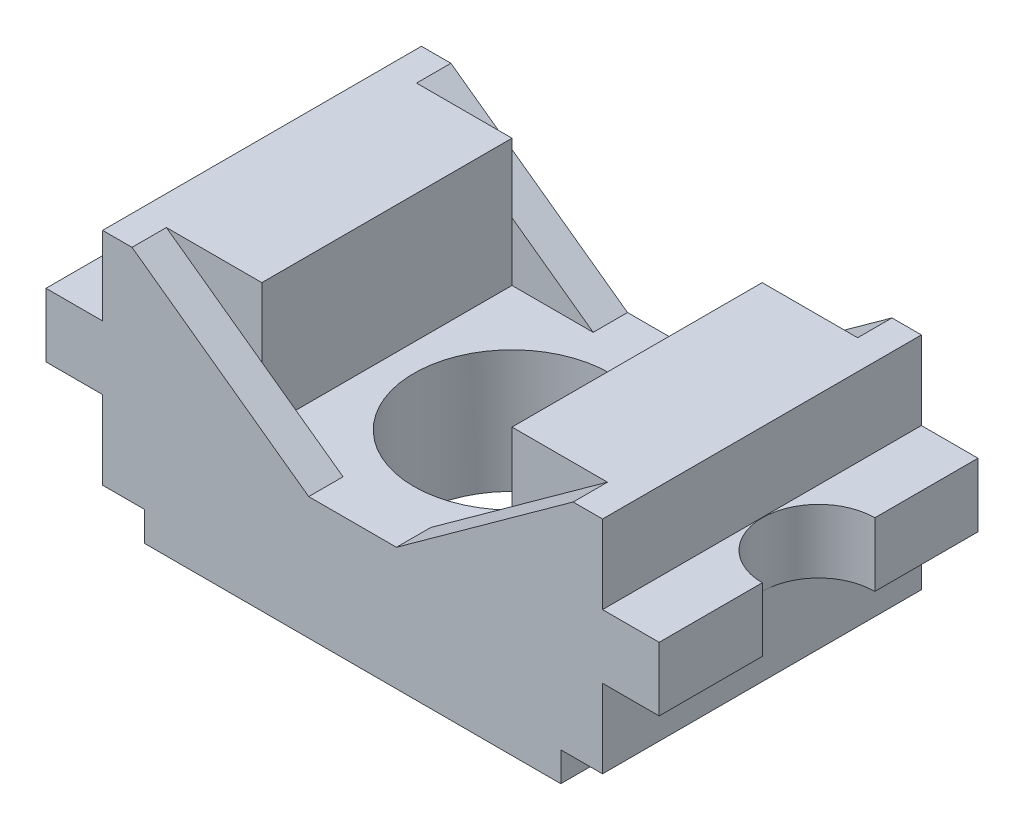
ISO-10303-21;
HEADER;
FILE_DESCRIPTION(('STEP AP214'),'2;1');
FILE_NAME('part.step','',(''),(''),'','','');
FILE_SCHEMA(('AUTOMOTIVE_DESIGN { 1 0 10303 214 1 1 1 1 }'));
ENDSEC;
DATA;
#1=APPLICATION_CONTEXT('core data for automotive mechanical design processes');
#2=APPLICATION_PROTOCOL_DEFINITION('international standard','automotive_design',2000,#1);
#3=PRODUCT_CONTEXT('',#1,'mechanical');
#4=PRODUCT('Part','Part','',(#3));
#5=PRODUCT_RELATED_PRODUCT_CATEGORY('part','',(#4));
#6=PRODUCT_DEFINITION_FORMATION('','',#4);
#7=PRODUCT_DEFINITION_CONTEXT('part definition',#1,'design');
#8=PRODUCT_DEFINITION('design','',#6,#7);
#9=PRODUCT_DEFINITION_SHAPE('','',#8);
#10=(LENGTH_UNIT() NAMED_UNIT(*) SI_UNIT(.MILLI.,.METRE.));
#11=(NAMED_UNIT(*) PLANE_ANGLE_UNIT() SI_UNIT($,.RADIAN.));
#12=(NAMED_UNIT(*) SI_UNIT($,.STERADIAN.) SOLID_ANGLE_UNIT());
#13=UNCERTAINTY_MEASURE_WITH_UNIT(LENGTH_MEASURE(1.E-05),#10,'distance_accuracy_value','');
#14=(GEOMETRIC_REPRESENTATION_CONTEXT(3) GLOBAL_UNCERTAINTY_ASSIGNED_CONTEXT((#13)) GLOBAL_UNIT_ASSIGNED_CONTEXT((#10,
#11,#12)) REPRESENTATION_CONTEXT('',''));
#15=CARTESIAN_POINT('',(0.,0.,0.));
#16=DIRECTION('',(0.,0.,1.));
#17=DIRECTION('',(1.,0.,0.));
#18=AXIS2_PLACEMENT_3D('',#15,#16,#17);
#19=CARTESIAN_POINT('',(62.5,22.,-65.));
#20=DIRECTION('',(1.,0.,0.));
#21=DIRECTION('',(0.,0.,-1.));
#22=AXIS2_PLACEMENT_3D('',#19,#20,#21);
#23=PLANE('',#22);
#24=DIRECTION('',(0.,1.,0.));
#25=VECTOR('',#24,1.);
#26=CARTESIAN_POINT('',(62.5,-6.00000000000003,-43.9726799835102));
#27=LINE('',#26,#25);
#28=CARTESIAN_POINT('',(62.5,22.,-43.9726799835102));
#29=VERTEX_POINT('',#28);
#30=CARTESIAN_POINT('',(62.5,35.,-43.9726799835102));
#31=VERTEX_POINT('',#30);
#32=EDGE_CURVE('E358',#29,#31,#27,.T.);
#33=ORIENTED_EDGE('',*,*,#32,.F.);
#34=DIRECTION('',(0.,0.,1.));
#35=VECTOR('',#34,1.);
#36=CARTESIAN_POINT('',(62.5,22.,-65.));
#37=LINE('',#36,#35);
#38=CARTESIAN_POINT('',(62.5,22.,-65.));
#39=VERTEX_POINT('',#38);
#40=EDGE_CURVE('E309',#39,#29,#37,.T.);
#41=ORIENTED_EDGE('',*,*,#40,.F.);
#42=DIRECTION('',(0.,1.,0.));
#43=VECTOR('',#42,1.);
#44=CARTESIAN_POINT('',(62.5,22.,-65.));
#45=LINE('',#44,#43);
#46=CARTESIAN_POINT('',(62.5,35.,-65.));
#47=VERTEX_POINT('',#46);
#48=EDGE_CURVE('E441',#39,#47,#45,.T.);
#49=ORIENTED_EDGE('',*,*,#48,.T.);
#50=DIRECTION('',(0.,0.,1.));
#51=VECTOR('',#50,1.);
#52=CARTESIAN_POINT('',(62.5,35.,-65.));
#53=LINE('',#52,#51);
#54=EDGE_CURVE('E313',#47,#31,#53,.T.);
#55=ORIENTED_EDGE('',*,*,#54,.T.);
#56=EDGE_LOOP('',(#33,#41,#49,#55));
#57=FACE_BOUND('',#56,.T.);
#58=ADVANCED_FACE('F39',(#57),#23,.T.);
#59=CARTESIAN_POINT('',(-62.5,22.,-65.));
#60=DIRECTION('',(1.,0.,0.));
#61=DIRECTION('',(0.,0.,-1.));
#62=AXIS2_PLACEMENT_3D('',#59,#60,#61);
#63=PLANE('',#62);
#64=DIRECTION('',(0.,0.,1.));
#65=VECTOR('',#64,1.);
#66=CARTESIAN_POINT('',(-62.5,22.,-65.));
#67=LINE('',#66,#65);
#68=CARTESIAN_POINT('',(-62.5,22.,-65.));
#69=VERTEX_POINT('',#68);
#70=CARTESIAN_POINT('',(-62.5,22.,-43.9918315677256));
#71=VERTEX_POINT('',#70);
#72=EDGE_CURVE('E274',#69,#71,#67,.T.);
#73=ORIENTED_EDGE('',*,*,#72,.T.);
#74=DIRECTION('',(0.,1.,0.));
#75=VECTOR('',#74,1.);
#76=CARTESIAN_POINT('',(-62.5,-6.00000000000003,-43.9918315677256));
#77=LINE('',#76,#75);
#78=CARTESIAN_POINT('',(-62.5,35.,-43.9918315677256));
#79=VERTEX_POINT('',#78);
#80=EDGE_CURVE('E256',#71,#79,#77,.T.);
#81=ORIENTED_EDGE('',*,*,#80,.T.);
#82=DIRECTION('',(0.,0.,1.));
#83=VECTOR('',#82,1.);
#84=CARTESIAN_POINT('',(-62.5,35.,-65.));
#85=LINE('',#84,#83);
#86=CARTESIAN_POINT('',(-62.5,35.,-65.));
#87=VERTEX_POINT('',#86);
#88=EDGE_CURVE('E272',#87,#79,#85,.T.);
#89=ORIENTED_EDGE('',*,*,#88,.F.);
#90=DIRECTION('',(0.,1.,0.));
#91=VECTOR('',#90,1.);
#92=CARTESIAN_POINT('',(-62.5,22.,-65.));
#93=LINE('',#92,#91);
#94=EDGE_CURVE('E470',#69,#87,#93,.T.);
#95=ORIENTED_EDGE('',*,*,#94,.F.);
#96=EDGE_LOOP('',(#73,#81,#89,#95));
#97=FACE_BOUND('',#96,.T.);
#98=ADVANCED_FACE('F268',(#97),#63,.F.);
#99=CARTESIAN_POINT('',(-44.9603846752662,51.,-65.));
#100=DIRECTION('',(-0.585334651975504,-0.810791801387209,0.));
#101=DIRECTION('',(0.810791801387209,-0.585334651975504,0.));
#102=AXIS2_PLACEMENT_3D('',#99,#100,#101);
#103=PLANE('',#102);
#104=DIRECTION('',(0.810791801387209,-0.585334651975504,0.));
#105=VECTOR('',#104,1.);
#106=CARTESIAN_POINT('',(-44.9603846752662,51.,-7.00000000000001));
#107=LINE('',#106,#105);
#108=CARTESIAN_POINT('',(-25.5,36.9509710486497,-7.00000000000001));
#109=VERTEX_POINT('',#108);
#110=CARTESIAN_POINT('',(-8.94579581584967,25.,-7.00000000000001));
#111=VERTEX_POINT('',#110);
#112=EDGE_CURVE('E389',#109,#111,#107,.T.);
#113=ORIENTED_EDGE('',*,*,#112,.F.);
#114=DIRECTION('',(0.810791801387209,-0.585334651975504,0.));
#115=VECTOR('',#114,1.);
#116=CARTESIAN_POINT('',(-44.9603846752662,51.,-7.00000000000001));
#117=LINE('',#116,#115);
#118=CARTESIAN_POINT('',(-44.9603846752661,51.,-7.00000000000001));
#119=VERTEX_POINT('',#118);
#120=EDGE_CURVE('E345',#119,#109,#117,.T.);
#121=ORIENTED_EDGE('',*,*,#120,.F.);
#122=DIRECTION('',(0.,0.,1.));
#123=VECTOR('',#122,1.);
#124=CARTESIAN_POINT('',(-44.9603846752662,51.,-65.));
#125=LINE('',#124,#123);
#126=CARTESIAN_POINT('',(-44.9603846752662,51.,0.));
#127=VERTEX_POINT('',#126);
#128=EDGE_CURVE('E335',#119,#127,#125,.T.);
#129=ORIENTED_EDGE('',*,*,#128,.T.);
#130=DIRECTION('',(0.810791801387209,-0.585334651975504,0.));
#131=VECTOR('',#130,1.);
#132=CARTESIAN_POINT('',(-44.9603846752662,51.,0.));
#133=LINE('',#132,#131);
#134=CARTESIAN_POINT('',(-8.94579581584967,25.,0.));
#135=VERTEX_POINT('',#134);
#136=EDGE_CURVE('E473',#127,#135,#133,.T.);
#137=ORIENTED_EDGE('',*,*,#136,.T.);
#138=DIRECTION('',(0.,0.,1.));
#139=VECTOR('',#138,1.);
#140=CARTESIAN_POINT('',(-8.94579581584967,25.,-65.));
#141=LINE('',#140,#139);
#142=EDGE_CURVE('E328',#111,#135,#141,.T.);
#143=ORIENTED_EDGE('',*,*,#142,.F.);
#144=EDGE_LOOP('',(#113,#121,#129,#137,#143));
#145=FACE_BOUND('',#144,.T.);
#146=ADVANCED_FACE('F543',(#145),#103,.F.);
#147=DIRECTION('',(-0.810791801387209,0.585334651975504,0.));
#148=VECTOR('',#147,1.);
#149=CARTESIAN_POINT('',(-44.9603846752662,51.,-58.));
#150=LINE('',#149,#148);
#151=CARTESIAN_POINT('',(-8.94579581584967,25.,-58.));
#152=VERTEX_POINT('',#151);
#153=CARTESIAN_POINT('',(-25.5,36.9509710486497,-58.));
#154=VERTEX_POINT('',#153);
#155=EDGE_CURVE('E384',#152,#154,#150,.T.);
#156=ORIENTED_EDGE('',*,*,#155,.F.);
#157=CARTESIAN_POINT('',(-8.94579581584967,25.,-65.));
#158=VERTEX_POINT('',#157);
#159=EDGE_CURVE('E330',#158,#152,#141,.T.);
#160=ORIENTED_EDGE('',*,*,#159,.F.);
#161=DIRECTION('',(0.810791801387209,-0.585334651975504,0.));
#162=VECTOR('',#161,1.);
#163=CARTESIAN_POINT('',(-44.9603846752662,51.,-65.));
#164=LINE('',#163,#162);
#165=CARTESIAN_POINT('',(-44.9603846752662,51.,-65.));
#166=VERTEX_POINT('',#165);
#167=EDGE_CURVE('E425',#166,#158,#164,.T.);
#168=ORIENTED_EDGE('',*,*,#167,.F.);
#169=CARTESIAN_POINT('',(-44.9603846752662,51.,-58.));
#170=VERTEX_POINT('',#169);
#171=EDGE_CURVE('E333',#166,#170,#125,.T.);
#172=ORIENTED_EDGE('',*,*,#171,.T.);
#173=DIRECTION('',(-0.810791801387209,0.585334651975504,0.));
#174=VECTOR('',#173,1.);
#175=CARTESIAN_POINT('',(-44.9603846752662,51.,-58.));
#176=LINE('',#175,#174);
#177=EDGE_CURVE('E50',#154,#170,#176,.T.);
#178=ORIENTED_EDGE('',*,*,#177,.F.);
#179=EDGE_LOOP('',(#156,#160,#168,#172,#178));
#180=FACE_BOUND('',#179,.T.);
#181=ADVANCED_FACE('F559',(#180),#103,.F.);
#182=CARTESIAN_POINT('',(44.9603846752662,51.,-65.));
#183=DIRECTION('',(-0.585334651975504,0.810791801387209,0.));
#184=DIRECTION('',(-0.810791801387209,-0.585334651975504,0.));
#185=AXIS2_PLACEMENT_3D('',#182,#183,#184);
#186=PLANE('',#185);
#187=DIRECTION('',(-0.810791801387209,-0.585334651975504,0.));
#188=VECTOR('',#187,1.);
#189=CARTESIAN_POINT('',(44.9603846752662,51.,-7.00000000000001));
#190=LINE('',#189,#188);
#191=CARTESIAN_POINT('',(44.9603846752662,51.,-7.00000000000001));
#192=VERTEX_POINT('',#191);
#193=CARTESIAN_POINT('',(25.5,36.9509710486497,-7.00000000000001));
#194=VERTEX_POINT('',#193);
#195=EDGE_CURVE('E339',#192,#194,#190,.T.);
#196=ORIENTED_EDGE('',*,*,#195,.T.);
#197=DIRECTION('',(-0.810791801387209,-0.585334651975504,0.));
#198=VECTOR('',#197,1.);
#199=CARTESIAN_POINT('',(44.9603846752662,51.,-7.00000000000001));
#200=LINE('',#199,#198);
#201=CARTESIAN_POINT('',(8.94579581584967,25.,-7.00000000000001));
#202=VERTEX_POINT('',#201);
#203=EDGE_CURVE('E383',#194,#202,#200,.T.);
#204=ORIENTED_EDGE('',*,*,#203,.T.);
#205=DIRECTION('',(0.,0.,1.));
#206=VECTOR('',#205,1.);
#207=CARTESIAN_POINT('',(8.94579581584967,25.,-65.));
#208=LINE('',#207,#206);
#209=CARTESIAN_POINT('',(8.94579581584967,25.,0.));
#210=VERTEX_POINT('',#209);
#211=EDGE_CURVE('E323',#202,#210,#208,.T.);
#212=ORIENTED_EDGE('',*,*,#211,.T.);
#213=DIRECTION('',(-0.810791801387209,-0.585334651975504,0.));
#214=VECTOR('',#213,1.);
#215=CARTESIAN_POINT('',(44.9603846752662,51.,0.));
#216=LINE('',#215,#214);
#217=CARTESIAN_POINT('',(44.9603846752662,51.,0.));
#218=VERTEX_POINT('',#217);
#219=EDGE_CURVE('E484',#218,#210,#216,.T.);
#220=ORIENTED_EDGE('',*,*,#219,.F.);
#221=DIRECTION('',(0.,0.,1.));
#222=VECTOR('',#221,1.);
#223=CARTESIAN_POINT('',(44.9603846752662,51.,-65.));
#224=LINE('',#223,#222);
#225=EDGE_CURVE('E322',#192,#218,#224,.T.);
#226=ORIENTED_EDGE('',*,*,#225,.F.);
#227=EDGE_LOOP('',(#196,#204,#212,#220,#226));
#228=FACE_BOUND('',#227,.T.);
#229=ADVANCED_FACE('F603',(#228),#186,.T.);
#230=CARTESIAN_POINT('',(8.94579581584967,25.,-65.));
#231=VERTEX_POINT('',#230);
#232=CARTESIAN_POINT('',(8.94579581584967,25.,-58.));
#233=VERTEX_POINT('',#232);
#234=EDGE_CURVE('E326',#231,#233,#208,.T.);
#235=ORIENTED_EDGE('',*,*,#234,.T.);
#236=DIRECTION('',(0.810791801387209,0.585334651975504,0.));
#237=VECTOR('',#236,1.);
#238=CARTESIAN_POINT('',(44.9603846752662,51.,-58.));
#239=LINE('',#238,#237);
#240=CARTESIAN_POINT('',(25.5,36.9509710486497,-58.));
#241=VERTEX_POINT('',#240);
#242=EDGE_CURVE('E379',#233,#241,#239,.T.);
#243=ORIENTED_EDGE('',*,*,#242,.T.);
#244=DIRECTION('',(0.810791801387209,0.585334651975504,0.));
#245=VECTOR('',#244,1.);
#246=CARTESIAN_POINT('',(44.9603846752662,51.,-58.));
#247=LINE('',#246,#245);
#248=CARTESIAN_POINT('',(44.9603846752662,51.,-58.));
#249=VERTEX_POINT('',#248);
#250=EDGE_CURVE('E337',#241,#249,#247,.T.);
#251=ORIENTED_EDGE('',*,*,#250,.T.);
#252=CARTESIAN_POINT('',(44.9603846752662,51.,-65.));
#253=VERTEX_POINT('',#252);
#254=EDGE_CURVE('E325',#253,#249,#224,.T.);
#255=ORIENTED_EDGE('',*,*,#254,.F.);
#256=DIRECTION('',(-0.810791801387209,-0.585334651975504,0.));
#257=VECTOR('',#256,1.);
#258=CARTESIAN_POINT('',(44.9603846752662,51.,-65.));
#259=LINE('',#258,#257);
#260=EDGE_CURVE('E429',#253,#231,#259,.T.);
#261=ORIENTED_EDGE('',*,*,#260,.T.);
#262=EDGE_LOOP('',(#235,#243,#251,#255,#261));
#263=FACE_BOUND('',#262,.T.);
#264=ADVANCED_FACE('F620',(#263),#186,.T.);
#265=CARTESIAN_POINT('',(-50.9603846752662,51.,-65.));
#266=DIRECTION('',(0.,-1.,0.));
#267=DIRECTION('',(0.,0.,-1.));
#268=AXIS2_PLACEMENT_3D('',#265,#266,#267);
#269=PLANE('',#268);
#270=DIRECTION('',(1.,0.,0.));
#271=VECTOR('',#270,1.);
#272=CARTESIAN_POINT('',(-50.9603846752662,51.,0.));
#273=LINE('',#272,#271);
#274=CARTESIAN_POINT('',(-50.9603846752662,51.,0.));
#275=VERTEX_POINT('',#274);
#276=EDGE_CURVE('E398',#275,#127,#273,.T.);
#277=ORIENTED_EDGE('',*,*,#276,.T.);
#278=ORIENTED_EDGE('',*,*,#128,.F.);
#279=DIRECTION('',(-1.,0.,0.));
#280=VECTOR('',#279,1.);
#281=CARTESIAN_POINT('',(-44.9603846752661,51.,-7.00000000000001));
#282=LINE('',#281,#280);
#283=CARTESIAN_POINT('',(-25.5,51.,-7.00000000000001));
#284=VERTEX_POINT('',#283);
#285=EDGE_CURVE('E395',#284,#119,#282,.T.);
#286=ORIENTED_EDGE('',*,*,#285,.F.);
#287=DIRECTION('',(0.,0.,1.));
#288=VECTOR('',#287,1.);
#289=CARTESIAN_POINT('',(-25.5,51.,-58.));
#290=LINE('',#289,#288);
#291=CARTESIAN_POINT('',(-25.5,51.,-58.));
#292=VERTEX_POINT('',#291);
#293=EDGE_CURVE('E392',#292,#284,#290,.T.);
#294=ORIENTED_EDGE('',*,*,#293,.F.);
#295=DIRECTION('',(1.,0.,0.));
#296=VECTOR('',#295,1.);
#297=CARTESIAN_POINT('',(-44.9603846752662,51.,-58.));
#298=LINE('',#297,#296);
#299=EDGE_CURVE('E399',#170,#292,#298,.T.);
#300=ORIENTED_EDGE('',*,*,#299,.F.);
#301=ORIENTED_EDGE('',*,*,#171,.F.);
#302=DIRECTION('',(1.,0.,0.));
#303=VECTOR('',#302,1.);
#304=CARTESIAN_POINT('',(-50.9603846752662,51.,-65.));
#305=LINE('',#304,#303);
#306=CARTESIAN_POINT('',(-50.9603846752662,51.,-65.));
#307=VERTEX_POINT('',#306);
#308=EDGE_CURVE('E423',#307,#166,#305,.T.);
#309=ORIENTED_EDGE('',*,*,#308,.F.);
#310=DIRECTION('',(0.,0.,1.));
#311=VECTOR('',#310,1.);
#312=CARTESIAN_POINT('',(-50.9603846752662,51.,-65.));
#313=LINE('',#312,#311);
#314=EDGE_CURVE('E475',#307,#275,#313,.T.);
#315=ORIENTED_EDGE('',*,*,#314,.T.);
#316=EDGE_LOOP('',(#277,#278,#286,#294,#300,#301,#309,#315));
#317=FACE_BOUND('',#316,.T.);
#318=ADVANCED_FACE('F41',(#317),#269,.F.);
#319=CARTESIAN_POINT('',(-8.94579581584967,25.,-65.));
#320=DIRECTION('',(0.,-1.,0.));
#321=DIRECTION('',(0.,0.,-1.));
#322=AXIS2_PLACEMENT_3D('',#319,#320,#321);
#323=PLANE('',#322);
#324=CARTESIAN_POINT('',(0.,25.,-32.5));
#325=DIRECTION('',(0.,1.,0.));
#326=DIRECTION('',(0.,0.,1.));
#327=AXIS2_PLACEMENT_3D('',#324,#325,#326);
#328=CIRCLE('',#327,20.);
#329=CARTESIAN_POINT('',(0.,25.,-12.5));
#330=VERTEX_POINT('',#329);
#331=EDGE_CURVE('E348',#330,#330,#328,.T.);
#332=ORIENTED_EDGE('',*,*,#331,.F.);
#333=EDGE_LOOP('',(#332));
#334=FACE_BOUND('',#333,.T.);
#335=ORIENTED_EDGE('',*,*,#159,.T.);
#336=DIRECTION('',(-1.,0.,0.));
#337=VECTOR('',#336,1.);
#338=CARTESIAN_POINT('',(-25.5,25.,-58.));
#339=LINE('',#338,#337);
#340=CARTESIAN_POINT('',(-25.5,25.,-58.));
#341=VERTEX_POINT('',#340);
#342=EDGE_CURVE('E368',#152,#341,#339,.T.);
#343=ORIENTED_EDGE('',*,*,#342,.T.);
#344=DIRECTION('',(0.,0.,1.));
#345=VECTOR('',#344,1.);
#346=CARTESIAN_POINT('',(-25.5,25.,-7.00000000000001));
#347=LINE('',#346,#345);
#348=CARTESIAN_POINT('',(-25.5,25.,-7.00000000000001));
#349=VERTEX_POINT('',#348);
#350=EDGE_CURVE('E349',#341,#349,#347,.T.);
#351=ORIENTED_EDGE('',*,*,#350,.T.);
#352=DIRECTION('',(1.,0.,0.));
#353=VECTOR('',#352,1.);
#354=CARTESIAN_POINT('',(-25.5,25.,-7.00000000000001));
#355=LINE('',#354,#353);
#356=EDGE_CURVE('E361',#349,#111,#355,.T.);
#357=ORIENTED_EDGE('',*,*,#356,.T.);
#358=ORIENTED_EDGE('',*,*,#142,.T.);
#359=DIRECTION('',(1.,0.,0.));
#360=VECTOR('',#359,1.);
#361=CARTESIAN_POINT('',(-8.94579581584967,25.,0.));
#362=LINE('',#361,#360);
#363=EDGE_CURVE('E479',#135,#210,#362,.T.);
#364=ORIENTED_EDGE('',*,*,#363,.T.);
#365=ORIENTED_EDGE('',*,*,#211,.F.);
#366=CARTESIAN_POINT('',(25.5,25.,-7.00000000000001));
#367=VERTEX_POINT('',#366);
#368=EDGE_CURVE('E355',#202,#367,#355,.T.);
#369=ORIENTED_EDGE('',*,*,#368,.T.);
#370=DIRECTION('',(0.,0.,-1.));
#371=VECTOR('',#370,1.);
#372=CARTESIAN_POINT('',(25.5,25.,-7.00000000000001));
#373=LINE('',#372,#371);
#374=CARTESIAN_POINT('',(25.5,25.,-58.));
#375=VERTEX_POINT('',#374);
#376=EDGE_CURVE('E362',#367,#375,#373,.T.);
#377=ORIENTED_EDGE('',*,*,#376,.T.);
#378=EDGE_CURVE('E367',#375,#233,#339,.T.);
#379=ORIENTED_EDGE('',*,*,#378,.T.);
#380=ORIENTED_EDGE('',*,*,#234,.F.);
#381=DIRECTION('',(1.,0.,0.));
#382=VECTOR('',#381,1.);
#383=CARTESIAN_POINT('',(-8.94579581584967,25.,-65.));
#384=LINE('',#383,#382);
#385=EDGE_CURVE('E430',#158,#231,#384,.T.);
#386=ORIENTED_EDGE('',*,*,#385,.F.);
#387=EDGE_LOOP('',(#335,#343,#351,#357,#358,#364,#365,#369,#377,#379,#380,#386));
#388=FACE_BOUND('',#387,.T.);
#389=ADVANCED_FACE('F608',(#334,#388),#323,.F.);
#390=CARTESIAN_POINT('',(50.9603846752662,51.,-65.));
#391=DIRECTION('',(0.,1.,0.));
#392=DIRECTION('',(0.,0.,1.));
#393=AXIS2_PLACEMENT_3D('',#390,#391,#392);
#394=PLANE('',#393);
#395=DIRECTION('',(-1.,0.,0.));
#396=VECTOR('',#395,1.);
#397=CARTESIAN_POINT('',(50.9603846752662,51.,0.));
#398=LINE('',#397,#396);
#399=CARTESIAN_POINT('',(50.9603846752662,51.,0.));
#400=VERTEX_POINT('',#399);
#401=EDGE_CURVE('E483',#400,#218,#398,.T.);
#402=ORIENTED_EDGE('',*,*,#401,.F.);
#403=DIRECTION('',(0.,0.,1.));
#404=VECTOR('',#403,1.);
#405=CARTESIAN_POINT('',(50.9603846752662,51.,-65.));
#406=LINE('',#405,#404);
#407=CARTESIAN_POINT('',(50.9603846752662,51.,-65.));
#408=VERTEX_POINT('',#407);
#409=EDGE_CURVE('E316',#408,#400,#406,.T.);
#410=ORIENTED_EDGE('',*,*,#409,.F.);
#411=DIRECTION('',(-1.,0.,0.));
#412=VECTOR('',#411,1.);
#413=CARTESIAN_POINT('',(50.9603846752662,51.,-65.));
#414=LINE('',#413,#412);
#415=EDGE_CURVE('E435',#408,#253,#414,.T.);
#416=ORIENTED_EDGE('',*,*,#415,.T.);
#417=ORIENTED_EDGE('',*,*,#254,.T.);
#418=DIRECTION('',(1.,0.,0.));
#419=VECTOR('',#418,1.);
#420=CARTESIAN_POINT('',(44.9603846752662,51.,-58.));
#421=LINE('',#420,#419);
#422=CARTESIAN_POINT('',(25.5,51.,-58.));
#423=VERTEX_POINT('',#422);
#424=EDGE_CURVE('E391',#423,#249,#421,.T.);
#425=ORIENTED_EDGE('',*,*,#424,.F.);
#426=DIRECTION('',(0.,0.,-1.));
#427=VECTOR('',#426,1.);
#428=CARTESIAN_POINT('',(25.5,51.,-58.));
#429=LINE('',#428,#427);
#430=CARTESIAN_POINT('',(25.5,51.,-7.00000000000001));
#431=VERTEX_POINT('',#430);
#432=EDGE_CURVE('E414',#431,#423,#429,.T.);
#433=ORIENTED_EDGE('',*,*,#432,.F.);
#434=DIRECTION('',(-1.,0.,0.));
#435=VECTOR('',#434,1.);
#436=CARTESIAN_POINT('',(44.9603846752661,51.,-7.00000000000001));
#437=LINE('',#436,#435);
#438=EDGE_CURVE('E406',#192,#431,#437,.T.);
#439=ORIENTED_EDGE('',*,*,#438,.F.);
#440=ORIENTED_EDGE('',*,*,#225,.T.);
#441=EDGE_LOOP('',(#402,#410,#416,#417,#425,#433,#439,#440));
#442=FACE_BOUND('',#441,.T.);
#443=ADVANCED_FACE('F602',(#442),#394,.T.);
#444=CARTESIAN_POINT('',(50.9603846752662,35.,-65.));
#445=DIRECTION('',(1.,0.,0.));
#446=DIRECTION('',(0.,0.,-1.));
#447=AXIS2_PLACEMENT_3D('',#444,#445,#446);
#448=PLANE('',#447);
#449=DIRECTION('',(0.,1.,0.));
#450=VECTOR('',#449,1.);
#451=CARTESIAN_POINT('',(50.9603846752662,35.,0.));
#452=LINE('',#451,#450);
#453=CARTESIAN_POINT('',(50.9603846752662,35.,0.));
#454=VERTEX_POINT('',#453);
#455=EDGE_CURVE('E487',#454,#400,#452,.T.);
#456=ORIENTED_EDGE('',*,*,#455,.F.);
#457=DIRECTION('',(0.,0.,1.));
#458=VECTOR('',#457,1.);
#459=CARTESIAN_POINT('',(50.9603846752662,35.,-65.));
#460=LINE('',#459,#458);
#461=CARTESIAN_POINT('',(50.9603846752662,35.,-65.));
#462=VERTEX_POINT('',#461);
#463=EDGE_CURVE('E320',#462,#454,#460,.T.);
#464=ORIENTED_EDGE('',*,*,#463,.F.);
#465=DIRECTION('',(0.,1.,0.));
#466=VECTOR('',#465,1.);
#467=CARTESIAN_POINT('',(50.9603846752662,35.,-65.));
#468=LINE('',#467,#466);
#469=EDGE_CURVE('E434',#462,#408,#468,.T.);
#470=ORIENTED_EDGE('',*,*,#469,.T.);
#471=ORIENTED_EDGE('',*,*,#409,.T.);
#472=EDGE_LOOP('',(#456,#464,#470,#471));
#473=FACE_BOUND('',#472,.T.);
#474=ADVANCED_FACE('F600',(#473),#448,.T.);
#475=CARTESIAN_POINT('',(62.5,35.,-65.));
#476=DIRECTION('',(0.,1.,0.));
#477=DIRECTION('',(0.,0.,1.));
#478=AXIS2_PLACEMENT_3D('',#475,#476,#477);
#479=PLANE('',#478);
#480=CARTESIAN_POINT('',(62.5,35.,-32.5));
#481=DIRECTION('',(0.,1.,0.));
#482=DIRECTION('',(0.,0.,1.));
#483=AXIS2_PLACEMENT_3D('',#480,#481,#482);
#484=CIRCLE('',#483,11.4726799835102);
#485=CARTESIAN_POINT('',(62.5,35.,-21.0273200164898));
#486=VERTEX_POINT('',#485);
#487=EDGE_CURVE('E263',#31,#486,#484,.T.);
#488=ORIENTED_EDGE('',*,*,#487,.F.);
#489=ORIENTED_EDGE('',*,*,#54,.F.);
#490=DIRECTION('',(-1.,0.,0.));
#491=VECTOR('',#490,1.);
#492=CARTESIAN_POINT('',(62.5,35.,-65.));
#493=LINE('',#492,#491);
#494=EDGE_CURVE('E438',#47,#462,#493,.T.);
#495=ORIENTED_EDGE('',*,*,#494,.T.);
#496=ORIENTED_EDGE('',*,*,#463,.T.);
#497=DIRECTION('',(-1.,0.,0.));
#498=VECTOR('',#497,1.);
#499=CARTESIAN_POINT('',(62.5,35.,0.));
#500=LINE('',#499,#498);
#501=CARTESIAN_POINT('',(62.5,35.,0.));
#502=VERTEX_POINT('',#501);
#503=EDGE_CURVE('E489',#502,#454,#500,.T.);
#504=ORIENTED_EDGE('',*,*,#503,.F.);
#505=EDGE_CURVE('E312',#486,#502,#53,.T.);
#506=ORIENTED_EDGE('',*,*,#505,.F.);
#507=EDGE_LOOP('',(#488,#489,#495,#496,#504,#506));
#508=FACE_BOUND('',#507,.T.);
#509=ADVANCED_FACE('F584',(#508),#479,.T.);
#510=DIRECTION('',(0.,1.,0.));
#511=VECTOR('',#510,1.);
#512=CARTESIAN_POINT('',(62.5,-6.00000000000003,-21.0273200164898));
#513=LINE('',#512,#511);
#514=CARTESIAN_POINT('',(62.5,22.,-21.0273200164898));
#515=VERTEX_POINT('',#514);
#516=EDGE_CURVE('E52',#486,#515,#513,.F.);
#517=ORIENTED_EDGE('',*,*,#516,.F.);
#518=ORIENTED_EDGE('',*,*,#505,.T.);
#519=DIRECTION('',(0.,1.,0.));
#520=VECTOR('',#519,1.);
#521=CARTESIAN_POINT('',(62.5,22.,0.));
#522=LINE('',#521,#520);
#523=CARTESIAN_POINT('',(62.5,22.,0.));
#524=VERTEX_POINT('',#523);
#525=EDGE_CURVE('E491',#524,#502,#522,.T.);
#526=ORIENTED_EDGE('',*,*,#525,.F.);
#527=EDGE_CURVE('E307',#515,#524,#37,.T.);
#528=ORIENTED_EDGE('',*,*,#527,.F.);
#529=EDGE_LOOP('',(#517,#518,#526,#528));
#530=FACE_BOUND('',#529,.T.);
#531=ADVANCED_FACE('F578',(#530),#23,.T.);
#532=CARTESIAN_POINT('',(50.9603846752661,22.,-65.));
#533=DIRECTION('',(0.,-1.,0.));
#534=DIRECTION('',(0.,0.,-1.));
#535=AXIS2_PLACEMENT_3D('',#532,#533,#534);
#536=PLANE('',#535);
#537=CARTESIAN_POINT('',(62.5,22.,-32.5));
#538=DIRECTION('',(0.,-1.,0.));
#539=DIRECTION('',(0.,0.,-1.));
#540=AXIS2_PLACEMENT_3D('',#537,#538,#539);
#541=CIRCLE('',#540,11.4726799835102);
#542=EDGE_CURVE('E11',#515,#29,#541,.T.);
#543=ORIENTED_EDGE('',*,*,#542,.F.);
#544=ORIENTED_EDGE('',*,*,#527,.T.);
#545=DIRECTION('',(1.,0.,0.));
#546=VECTOR('',#545,1.);
#547=CARTESIAN_POINT('',(50.9603846752661,22.,0.));
#548=LINE('',#547,#546);
#549=CARTESIAN_POINT('',(50.9603846752661,22.,0.));
#550=VERTEX_POINT('',#549);
#551=EDGE_CURVE('E496',#550,#524,#548,.T.);
#552=ORIENTED_EDGE('',*,*,#551,.F.);
#553=DIRECTION('',(0.,0.,1.));
#554=VECTOR('',#553,1.);
#555=CARTESIAN_POINT('',(50.9603846752661,22.,-65.));
#556=LINE('',#555,#554);
#557=CARTESIAN_POINT('',(50.9603846752661,22.,-65.));
#558=VERTEX_POINT('',#557);
#559=EDGE_CURVE('E310',#558,#550,#556,.T.);
#560=ORIENTED_EDGE('',*,*,#559,.F.);
#561=DIRECTION('',(1.,0.,0.));
#562=VECTOR('',#561,1.);
#563=CARTESIAN_POINT('',(50.9603846752661,22.,-65.));
#564=LINE('',#563,#562);
#565=EDGE_CURVE('E443',#558,#39,#564,.T.);
#566=ORIENTED_EDGE('',*,*,#565,.T.);
#567=ORIENTED_EDGE('',*,*,#40,.T.);
#568=EDGE_LOOP('',(#543,#544,#552,#560,#566,#567));
#569=FACE_BOUND('',#568,.T.);
#570=ADVANCED_FACE('F589',(#569),#536,.T.);
#571=CARTESIAN_POINT('',(50.9603846752662,5.99999999999999,-65.));
#572=DIRECTION('',(1.,0.,0.));
#573=DIRECTION('',(0.,1.,0.));
#574=AXIS2_PLACEMENT_3D('',#571,#572,#573);
#575=PLANE('',#574);
#576=DIRECTION('',(0.,1.,0.));
#577=VECTOR('',#576,1.);
#578=CARTESIAN_POINT('',(50.9603846752662,5.99999999999999,0.));
#579=LINE('',#578,#577);
#580=CARTESIAN_POINT('',(50.9603846752662,5.99999999999999,0.));
#581=VERTEX_POINT('',#580);
#582=EDGE_CURVE('E497',#581,#550,#579,.T.);
#583=ORIENTED_EDGE('',*,*,#582,.F.);
#584=DIRECTION('',(0.,0.,1.));
#585=VECTOR('',#584,1.);
#586=CARTESIAN_POINT('',(50.9603846752662,5.99999999999999,-65.));
#587=LINE('',#586,#585);
#588=CARTESIAN_POINT('',(50.9603846752662,5.99999999999999,-65.));
#589=VERTEX_POINT('',#588);
#590=EDGE_CURVE('E304',#589,#581,#587,.T.);
#591=ORIENTED_EDGE('',*,*,#590,.F.);
#592=DIRECTION('',(0.,1.,0.));
#593=VECTOR('',#592,1.);
#594=CARTESIAN_POINT('',(50.9603846752662,5.99999999999999,-65.));
#595=LINE('',#594,#593);
#596=EDGE_CURVE('E450',#589,#558,#595,.T.);
#597=ORIENTED_EDGE('',*,*,#596,.T.);
#598=ORIENTED_EDGE('',*,*,#559,.T.);
#599=EDGE_LOOP('',(#583,#591,#597,#598));
#600=FACE_BOUND('',#599,.T.);
#601=ADVANCED_FACE('F659',(#600),#575,.T.);
#602=CARTESIAN_POINT('',(42.4457958158497,5.99999999999999,-65.));
#603=DIRECTION('',(0.,-1.,0.));
#604=DIRECTION('',(0.,0.,-1.));
#605=AXIS2_PLACEMENT_3D('',#602,#603,#604);
#606=PLANE('',#605);
#607=DIRECTION('',(1.,0.,0.));
#608=VECTOR('',#607,1.);
#609=CARTESIAN_POINT('',(42.4457958158497,5.99999999999999,0.));
#610=LINE('',#609,#608);
#611=CARTESIAN_POINT('',(42.4457958158497,5.99999999999999,0.));
#612=VERTEX_POINT('',#611);
#613=EDGE_CURVE('E505',#612,#581,#610,.T.);
#614=ORIENTED_EDGE('',*,*,#613,.F.);
#615=DIRECTION('',(0.,0.,1.));
#616=VECTOR('',#615,1.);
#617=CARTESIAN_POINT('',(42.4457958158497,5.99999999999999,-65.));
#618=LINE('',#617,#616);
#619=CARTESIAN_POINT('',(42.4457958158497,5.99999999999999,-65.));
#620=VERTEX_POINT('',#619);
#621=EDGE_CURVE('E303',#620,#612,#618,.T.);
#622=ORIENTED_EDGE('',*,*,#621,.F.);
#623=DIRECTION('',(1.,0.,0.));
#624=VECTOR('',#623,1.);
#625=CARTESIAN_POINT('',(42.4457958158497,5.99999999999999,-65.));
#626=LINE('',#625,#624);
#627=EDGE_CURVE('E448',#620,#589,#626,.T.);
#628=ORIENTED_EDGE('',*,*,#627,.T.);
#629=ORIENTED_EDGE('',*,*,#590,.T.);
#630=EDGE_LOOP('',(#614,#622,#628,#629));
#631=FACE_BOUND('',#630,.T.);
#632=ADVANCED_FACE('F950',(#631),#606,.T.);
#633=CARTESIAN_POINT('',(42.4457958158497,0.,-65.));
#634=DIRECTION('',(1.,0.,0.));
#635=DIRECTION('',(0.,0.,-1.));
#636=AXIS2_PLACEMENT_3D('',#633,#634,#635);
#637=PLANE('',#636);
#638=DIRECTION('',(0.,1.,0.));
#639=VECTOR('',#638,1.);
#640=CARTESIAN_POINT('',(42.4457958158497,0.,0.));
#641=LINE('',#640,#639);
#642=CARTESIAN_POINT('',(42.4457958158497,0.,0.));
#643=VERTEX_POINT('',#642);
#644=EDGE_CURVE('E504',#643,#612,#641,.T.);
#645=ORIENTED_EDGE('',*,*,#644,.F.);
#646=DIRECTION('',(0.,0.,1.));
#647=VECTOR('',#646,1.);
#648=CARTESIAN_POINT('',(42.4457958158497,0.,-65.));
#649=LINE('',#648,#647);
#650=CARTESIAN_POINT('',(42.4457958158497,0.,-65.));
#651=VERTEX_POINT('',#650);
#652=EDGE_CURVE('E297',#651,#643,#649,.T.);
#653=ORIENTED_EDGE('',*,*,#652,.F.);
#654=DIRECTION('',(0.,1.,0.));
#655=VECTOR('',#654,1.);
#656=CARTESIAN_POINT('',(42.4457958158497,0.,-65.));
#657=LINE('',#656,#655);
#658=EDGE_CURVE('E454',#651,#620,#657,.T.);
#659=ORIENTED_EDGE('',*,*,#658,.T.);
#660=ORIENTED_EDGE('',*,*,#621,.T.);
#661=EDGE_LOOP('',(#645,#653,#659,#660));
#662=FACE_BOUND('',#661,.T.);
#663=ADVANCED_FACE('F842',(#662),#637,.T.);
#664=CARTESIAN_POINT('',(-8.94579581584967,0.,-65.));
#665=DIRECTION('',(0.,1.,0.));
#666=DIRECTION('',(-1.,0.,0.));
#667=AXIS2_PLACEMENT_3D('',#664,#665,#666);
#668=PLANE('',#667);
#669=CARTESIAN_POINT('',(0.,0.,-32.5));
#670=DIRECTION('',(0.,1.,0.));
#671=DIRECTION('',(-1.,0.,0.));
#672=AXIS2_PLACEMENT_3D('',#669,#670,#671);
#673=CIRCLE('',#672,20.);
#674=CARTESIAN_POINT('',(-20.,0.,-32.5));
#675=VERTEX_POINT('',#674);
#676=EDGE_CURVE('E346',#675,#675,#673,.T.);
#677=ORIENTED_EDGE('',*,*,#676,.T.);
#678=EDGE_LOOP('',(#677));
#679=FACE_BOUND('',#678,.T.);
#680=DIRECTION('',(-1.,0.,0.));
#681=VECTOR('',#680,1.);
#682=CARTESIAN_POINT('',(-8.94579581584967,0.,0.));
#683=LINE('',#682,#681);
#684=CARTESIAN_POINT('',(-42.4457958158497,0.,0.));
#685=VERTEX_POINT('',#684);
#686=EDGE_CURVE('E507',#643,#685,#683,.T.);
#687=ORIENTED_EDGE('',*,*,#686,.T.);
#688=DIRECTION('',(0.,0.,1.));
#689=VECTOR('',#688,1.);
#690=CARTESIAN_POINT('',(-42.4457958158497,0.,-65.));
#691=LINE('',#690,#689);
#692=CARTESIAN_POINT('',(-42.4457958158497,0.,-65.));
#693=VERTEX_POINT('',#692);
#694=EDGE_CURVE('E300',#693,#685,#691,.T.);
#695=ORIENTED_EDGE('',*,*,#694,.F.);
#696=DIRECTION('',(1.,0.,0.));
#697=VECTOR('',#696,1.);
#698=CARTESIAN_POINT('',(8.94579581584967,0.,-65.));
#699=LINE('',#698,#697);
#700=EDGE_CURVE('E456',#693,#651,#699,.T.);
#701=ORIENTED_EDGE('',*,*,#700,.T.);
#702=ORIENTED_EDGE('',*,*,#652,.T.);
#703=EDGE_LOOP('',(#687,#695,#701,#702));
#704=FACE_BOUND('',#703,.T.);
#705=ADVANCED_FACE('F829',(#679,#704),#668,.F.);
#706=CARTESIAN_POINT('',(-42.4457958158497,0.,-65.));
#707=DIRECTION('',(1.,0.,0.));
#708=DIRECTION('',(0.,0.,-1.));
#709=AXIS2_PLACEMENT_3D('',#706,#707,#708);
#710=PLANE('',#709);
#711=DIRECTION('',(0.,1.,0.));
#712=VECTOR('',#711,1.);
#713=CARTESIAN_POINT('',(-42.4457958158497,0.,0.));
#714=LINE('',#713,#712);
#715=CARTESIAN_POINT('',(-42.4457958158497,5.99999999999999,0.));
#716=VERTEX_POINT('',#715);
#717=EDGE_CURVE('E509',#685,#716,#714,.T.);
#718=ORIENTED_EDGE('',*,*,#717,.T.);
#719=DIRECTION('',(0.,0.,1.));
#720=VECTOR('',#719,1.);
#721=CARTESIAN_POINT('',(-42.4457958158497,5.99999999999999,-65.));
#722=LINE('',#721,#720);
#723=CARTESIAN_POINT('',(-42.4457958158497,5.99999999999999,-65.));
#724=VERTEX_POINT('',#723);
#725=EDGE_CURVE('E295',#724,#716,#722,.T.);
#726=ORIENTED_EDGE('',*,*,#725,.F.);
#727=DIRECTION('',(0.,1.,0.));
#728=VECTOR('',#727,1.);
#729=CARTESIAN_POINT('',(-42.4457958158497,0.,-65.));
#730=LINE('',#729,#728);
#731=EDGE_CURVE('E458',#693,#724,#730,.T.);
#732=ORIENTED_EDGE('',*,*,#731,.F.);
#733=ORIENTED_EDGE('',*,*,#694,.T.);
#734=EDGE_LOOP('',(#718,#726,#732,#733));
#735=FACE_BOUND('',#734,.T.);
#736=ADVANCED_FACE('F817',(#735),#710,.F.);
#737=CARTESIAN_POINT('',(-42.4457958158497,5.99999999999999,-65.));
#738=DIRECTION('',(0.,1.,0.));
#739=DIRECTION('',(0.,0.,1.));
#740=AXIS2_PLACEMENT_3D('',#737,#738,#739);
#741=PLANE('',#740);
#742=DIRECTION('',(-1.,0.,0.));
#743=VECTOR('',#742,1.);
#744=CARTESIAN_POINT('',(-42.4457958158497,5.99999999999999,0.));
#745=LINE('',#744,#743);
#746=CARTESIAN_POINT('',(-50.9603846752662,5.99999999999999,0.));
#747=VERTEX_POINT('',#746);
#748=EDGE_CURVE('E515',#716,#747,#745,.T.);
#749=ORIENTED_EDGE('',*,*,#748,.T.);
#750=DIRECTION('',(0.,0.,1.));
#751=VECTOR('',#750,1.);
#752=CARTESIAN_POINT('',(-50.9603846752662,5.99999999999999,-65.));
#753=LINE('',#752,#751);
#754=CARTESIAN_POINT('',(-50.9603846752662,5.99999999999999,-65.));
#755=VERTEX_POINT('',#754);
#756=EDGE_CURVE('E293',#755,#747,#753,.T.);
#757=ORIENTED_EDGE('',*,*,#756,.F.);
#758=DIRECTION('',(-1.,0.,0.));
#759=VECTOR('',#758,1.);
#760=CARTESIAN_POINT('',(-42.4457958158497,5.99999999999999,-65.));
#761=LINE('',#760,#759);
#762=EDGE_CURVE('E464',#724,#755,#761,.T.);
#763=ORIENTED_EDGE('',*,*,#762,.F.);
#764=ORIENTED_EDGE('',*,*,#725,.T.);
#765=EDGE_LOOP('',(#749,#757,#763,#764));
#766=FACE_BOUND('',#765,.T.);
#767=ADVANCED_FACE('F807',(#766),#741,.F.);
#768=CARTESIAN_POINT('',(-50.9603846752662,5.99999999999999,-65.));
#769=DIRECTION('',(1.,0.,0.));
#770=DIRECTION('',(0.,1.,0.));
#771=AXIS2_PLACEMENT_3D('',#768,#769,#770);
#772=PLANE('',#771);
#773=DIRECTION('',(0.,1.,0.));
#774=VECTOR('',#773,1.);
#775=CARTESIAN_POINT('',(-50.9603846752662,5.99999999999999,0.));
#776=LINE('',#775,#774);
#777=CARTESIAN_POINT('',(-50.9603846752661,22.,0.));
#778=VERTEX_POINT('',#777);
#779=EDGE_CURVE('E511',#747,#778,#776,.T.);
#780=ORIENTED_EDGE('',*,*,#779,.T.);
#781=DIRECTION('',(0.,0.,1.));
#782=VECTOR('',#781,1.);
#783=CARTESIAN_POINT('',(-50.9603846752661,22.,-65.));
#784=LINE('',#783,#782);
#785=CARTESIAN_POINT('',(-50.9603846752661,22.,-65.));
#786=VERTEX_POINT('',#785);
#787=EDGE_CURVE('E290',#786,#778,#784,.T.);
#788=ORIENTED_EDGE('',*,*,#787,.F.);
#789=DIRECTION('',(0.,1.,0.));
#790=VECTOR('',#789,1.);
#791=CARTESIAN_POINT('',(-50.9603846752662,5.99999999999999,-65.));
#792=LINE('',#791,#790);
#793=EDGE_CURVE('E465',#755,#786,#792,.T.);
#794=ORIENTED_EDGE('',*,*,#793,.F.);
#795=ORIENTED_EDGE('',*,*,#756,.T.);
#796=EDGE_LOOP('',(#780,#788,#794,#795));
#797=FACE_BOUND('',#796,.T.);
#798=ADVANCED_FACE('F802',(#797),#772,.F.);
#799=CARTESIAN_POINT('',(-50.9603846752661,22.,-65.));
#800=DIRECTION('',(0.,1.,0.));
#801=DIRECTION('',(0.,0.,1.));
#802=AXIS2_PLACEMENT_3D('',#799,#800,#801);
#803=PLANE('',#802);
#804=CARTESIAN_POINT('',(-62.5,22.,-21.0081684322744));
#805=VERTEX_POINT('',#804);
#806=CARTESIAN_POINT('',(-62.5,22.,0.));
#807=VERTEX_POINT('',#806);
#808=EDGE_CURVE('E278',#805,#807,#67,.T.);
#809=ORIENTED_EDGE('',*,*,#808,.F.);
#810=CARTESIAN_POINT('',(-62.5,22.,-32.5));
#811=DIRECTION('',(0.,1.,0.));
#812=DIRECTION('',(0.,0.,1.));
#813=AXIS2_PLACEMENT_3D('',#810,#811,#812);
#814=CIRCLE('',#813,11.4918315677256);
#815=EDGE_CURVE('E273',#805,#71,#814,.T.);
#816=ORIENTED_EDGE('',*,*,#815,.T.);
#817=ORIENTED_EDGE('',*,*,#72,.F.);
#818=DIRECTION('',(-1.,0.,0.));
#819=VECTOR('',#818,1.);
#820=CARTESIAN_POINT('',(-50.9603846752661,22.,-65.));
#821=LINE('',#820,#819);
#822=EDGE_CURVE('E462',#786,#69,#821,.T.);
#823=ORIENTED_EDGE('',*,*,#822,.F.);
#824=ORIENTED_EDGE('',*,*,#787,.T.);
#825=DIRECTION('',(-1.,0.,0.));
#826=VECTOR('',#825,1.);
#827=CARTESIAN_POINT('',(-50.9603846752661,22.,0.));
#828=LINE('',#827,#826);
#829=EDGE_CURVE('E517',#778,#807,#828,.T.);
#830=ORIENTED_EDGE('',*,*,#829,.T.);
#831=EDGE_LOOP('',(#809,#816,#817,#823,#824,#830));
#832=FACE_BOUND('',#831,.T.);
#833=ADVANCED_FACE('F567',(#832),#803,.F.);
#834=CARTESIAN_POINT('',(-62.5,35.,-21.0081684322744));
#835=VERTEX_POINT('',#834);
#836=CARTESIAN_POINT('',(-62.5,35.,0.));
#837=VERTEX_POINT('',#836);
#838=EDGE_CURVE('E281',#835,#837,#85,.T.);
#839=ORIENTED_EDGE('',*,*,#838,.F.);
#840=DIRECTION('',(0.,1.,0.));
#841=VECTOR('',#840,1.);
#842=CARTESIAN_POINT('',(-62.5,-6.00000000000003,-21.0081684322744));
#843=LINE('',#842,#841);
#844=EDGE_CURVE('E62',#835,#805,#843,.F.);
#845=ORIENTED_EDGE('',*,*,#844,.T.);
#846=ORIENTED_EDGE('',*,*,#808,.T.);
#847=DIRECTION('',(0.,1.,0.));
#848=VECTOR('',#847,1.);
#849=CARTESIAN_POINT('',(-62.5,22.,0.));
#850=LINE('',#849,#848);
#851=EDGE_CURVE('E516',#807,#837,#850,.T.);
#852=ORIENTED_EDGE('',*,*,#851,.T.);
#853=EDGE_LOOP('',(#839,#845,#846,#852));
#854=FACE_BOUND('',#853,.T.);
#855=ADVANCED_FACE('F649',(#854),#63,.F.);
#856=CARTESIAN_POINT('',(-62.5,35.,-65.));
#857=DIRECTION('',(0.,-1.,0.));
#858=DIRECTION('',(0.,0.,-1.));
#859=AXIS2_PLACEMENT_3D('',#856,#857,#858);
#860=PLANE('',#859);
#861=ORIENTED_EDGE('',*,*,#88,.T.);
#862=CARTESIAN_POINT('',(-62.5,35.,-32.5));
#863=DIRECTION('',(0.,1.,0.));
#864=DIRECTION('',(0.,0.,1.));
#865=AXIS2_PLACEMENT_3D('',#862,#863,#864);
#866=CIRCLE('',#865,11.4918315677256);
#867=EDGE_CURVE('E257',#835,#79,#866,.T.);
#868=ORIENTED_EDGE('',*,*,#867,.F.);
#869=ORIENTED_EDGE('',*,*,#838,.T.);
#870=DIRECTION('',(1.,0.,0.));
#871=VECTOR('',#870,1.);
#872=CARTESIAN_POINT('',(-62.5,35.,0.));
#873=LINE('',#872,#871);
#874=CARTESIAN_POINT('',(-50.9603846752662,35.,0.));
#875=VERTEX_POINT('',#874);
#876=EDGE_CURVE('E522',#837,#875,#873,.T.);
#877=ORIENTED_EDGE('',*,*,#876,.T.);
#878=DIRECTION('',(0.,0.,1.));
#879=VECTOR('',#878,1.);
#880=CARTESIAN_POINT('',(-50.9603846752662,35.,-65.));
#881=LINE('',#880,#879);
#882=CARTESIAN_POINT('',(-50.9603846752662,35.,-65.));
#883=VERTEX_POINT('',#882);
#884=EDGE_CURVE('E283',#883,#875,#881,.T.);
#885=ORIENTED_EDGE('',*,*,#884,.F.);
#886=DIRECTION('',(1.,0.,0.));
#887=VECTOR('',#886,1.);
#888=CARTESIAN_POINT('',(-62.5,35.,-65.));
#889=LINE('',#888,#887);
#890=EDGE_CURVE('E276',#87,#883,#889,.T.);
#891=ORIENTED_EDGE('',*,*,#890,.F.);
#892=EDGE_LOOP('',(#861,#868,#869,#877,#885,#891));
#893=FACE_BOUND('',#892,.T.);
#894=ADVANCED_FACE('F280',(#893),#860,.F.);
#895=CARTESIAN_POINT('',(-50.9603846752662,35.,-65.));
#896=DIRECTION('',(1.,0.,0.));
#897=DIRECTION('',(0.,0.,-1.));
#898=AXIS2_PLACEMENT_3D('',#895,#896,#897);
#899=PLANE('',#898);
#900=DIRECTION('',(0.,1.,0.));
#901=VECTOR('',#900,1.);
#902=CARTESIAN_POINT('',(-50.9603846752662,35.,0.));
#903=LINE('',#902,#901);
#904=EDGE_CURVE('E424',#875,#275,#903,.T.);
#905=ORIENTED_EDGE('',*,*,#904,.T.);
#906=ORIENTED_EDGE('',*,*,#314,.F.);
#907=DIRECTION('',(0.,1.,0.));
#908=VECTOR('',#907,1.);
#909=CARTESIAN_POINT('',(-50.9603846752662,35.,-65.));
#910=LINE('',#909,#908);
#911=EDGE_CURVE('E468',#883,#307,#910,.T.);
#912=ORIENTED_EDGE('',*,*,#911,.F.);
#913=ORIENTED_EDGE('',*,*,#884,.T.);
#914=EDGE_LOOP('',(#905,#906,#912,#913));
#915=FACE_BOUND('',#914,.T.);
#916=ADVANCED_FACE('F531',(#915),#899,.F.);
#917=CARTESIAN_POINT('',(0.,0.,-65.));
#918=DIRECTION('',(0.,0.,1.));
#919=DIRECTION('',(1.,0.,0.));
#920=AXIS2_PLACEMENT_3D('',#917,#918,#919);
#921=PLANE('',#920);
#922=ORIENTED_EDGE('',*,*,#308,.T.);
#923=ORIENTED_EDGE('',*,*,#167,.T.);
#924=ORIENTED_EDGE('',*,*,#385,.T.);
#925=ORIENTED_EDGE('',*,*,#260,.F.);
#926=ORIENTED_EDGE('',*,*,#415,.F.);
#927=ORIENTED_EDGE('',*,*,#469,.F.);
#928=ORIENTED_EDGE('',*,*,#494,.F.);
#929=ORIENTED_EDGE('',*,*,#48,.F.);
#930=ORIENTED_EDGE('',*,*,#565,.F.);
#931=ORIENTED_EDGE('',*,*,#596,.F.);
#932=ORIENTED_EDGE('',*,*,#627,.F.);
#933=ORIENTED_EDGE('',*,*,#658,.F.);
#934=ORIENTED_EDGE('',*,*,#700,.F.);
#935=ORIENTED_EDGE('',*,*,#731,.T.);
#936=ORIENTED_EDGE('',*,*,#762,.T.);
#937=ORIENTED_EDGE('',*,*,#793,.T.);
#938=ORIENTED_EDGE('',*,*,#822,.T.);
#939=ORIENTED_EDGE('',*,*,#94,.T.);
#940=ORIENTED_EDGE('',*,*,#890,.T.);
#941=ORIENTED_EDGE('',*,*,#911,.T.);
#942=EDGE_LOOP('',(#922,#923,#924,#925,#926,#927,#928,#929,#930,#931,#932,#933,#934,#935,#936,
#937,#938,#939,#940,#941));
#943=FACE_BOUND('',#942,.T.);
#944=ADVANCED_FACE('F563',(#943),#921,.F.);
#945=CARTESIAN_POINT('',(0.,0.,0.));
#946=DIRECTION('',(0.,0.,1.));
#947=DIRECTION('',(1.,0.,0.));
#948=AXIS2_PLACEMENT_3D('',#945,#946,#947);
#949=PLANE('',#948);
#950=ORIENTED_EDGE('',*,*,#276,.F.);
#951=ORIENTED_EDGE('',*,*,#904,.F.);
#952=ORIENTED_EDGE('',*,*,#876,.F.);
#953=ORIENTED_EDGE('',*,*,#851,.F.);
#954=ORIENTED_EDGE('',*,*,#829,.F.);
#955=ORIENTED_EDGE('',*,*,#779,.F.);
#956=ORIENTED_EDGE('',*,*,#748,.F.);
#957=ORIENTED_EDGE('',*,*,#717,.F.);
#958=ORIENTED_EDGE('',*,*,#686,.F.);
#959=ORIENTED_EDGE('',*,*,#644,.T.);
#960=ORIENTED_EDGE('',*,*,#613,.T.);
#961=ORIENTED_EDGE('',*,*,#582,.T.);
#962=ORIENTED_EDGE('',*,*,#551,.T.);
#963=ORIENTED_EDGE('',*,*,#525,.T.);
#964=ORIENTED_EDGE('',*,*,#503,.T.);
#965=ORIENTED_EDGE('',*,*,#455,.T.);
#966=ORIENTED_EDGE('',*,*,#401,.T.);
#967=ORIENTED_EDGE('',*,*,#219,.T.);
#968=ORIENTED_EDGE('',*,*,#363,.F.);
#969=ORIENTED_EDGE('',*,*,#136,.F.);
#970=EDGE_LOOP('',(#950,#951,#952,#953,#954,#955,#956,#957,#958,#959,#960,#961,#962,#963,#964,
#965,#966,#967,#968,#969));
#971=FACE_BOUND('',#970,.T.);
#972=ADVANCED_FACE('F537',(#971),#949,.T.);
#973=CARTESIAN_POINT('',(44.9603846752661,105.586688594467,-7.00000000000001));
#974=DIRECTION('',(0.,0.,-1.));
#975=DIRECTION('',(-1.,0.,0.));
#976=AXIS2_PLACEMENT_3D('',#973,#974,#975);
#977=PLANE('',#976);
#978=ORIENTED_EDGE('',*,*,#195,.F.);
#979=ORIENTED_EDGE('',*,*,#438,.T.);
#980=DIRECTION('',(0.,-1.,0.));
#981=VECTOR('',#980,1.);
#982=CARTESIAN_POINT('',(25.5,105.586688594467,-7.00000000000001));
#983=LINE('',#982,#981);
#984=EDGE_CURVE('E404',#431,#194,#983,.T.);
#985=ORIENTED_EDGE('',*,*,#984,.T.);
#986=EDGE_LOOP('',(#978,#979,#985));
#987=FACE_BOUND('',#986,.T.);
#988=ADVANCED_FACE('F629',(#987),#977,.F.);
#989=CARTESIAN_POINT('',(25.5,105.586688594467,-58.));
#990=DIRECTION('',(1.,0.,0.));
#991=DIRECTION('',(0.,0.,-1.));
#992=AXIS2_PLACEMENT_3D('',#989,#990,#991);
#993=PLANE('',#992);
#994=DIRECTION('',(0.,-1.,0.));
#995=VECTOR('',#994,1.);
#996=CARTESIAN_POINT('',(25.5,105.586688594467,-58.));
#997=LINE('',#996,#995);
#998=EDGE_CURVE('E412',#423,#241,#997,.T.);
#999=ORIENTED_EDGE('',*,*,#998,.T.);
#1000=DIRECTION('',(0.,-1.,0.));
#1001=VECTOR('',#1000,1.);
#1002=CARTESIAN_POINT('',(25.5,66.,-58.));
#1003=LINE('',#1002,#1001);
#1004=EDGE_CURVE('E372',#241,#375,#1003,.T.);
#1005=ORIENTED_EDGE('',*,*,#1004,.T.);
#1006=ORIENTED_EDGE('',*,*,#376,.F.);
#1007=DIRECTION('',(0.,-1.,0.));
#1008=VECTOR('',#1007,1.);
#1009=CARTESIAN_POINT('',(25.5,66.,-7.00000000000001));
#1010=LINE('',#1009,#1008);
#1011=EDGE_CURVE('E376',#194,#367,#1010,.T.);
#1012=ORIENTED_EDGE('',*,*,#1011,.F.);
#1013=ORIENTED_EDGE('',*,*,#984,.F.);
#1014=ORIENTED_EDGE('',*,*,#432,.T.);
#1015=EDGE_LOOP('',(#999,#1005,#1006,#1012,#1013,#1014));
#1016=FACE_BOUND('',#1015,.T.);
#1017=ADVANCED_FACE('F622',(#1016),#993,.F.);
#1018=CARTESIAN_POINT('',(44.9603846752662,105.586688594467,-58.));
#1019=DIRECTION('',(0.,0.,1.));
#1020=DIRECTION('',(1.,0.,0.));
#1021=AXIS2_PLACEMENT_3D('',#1018,#1019,#1020);
#1022=PLANE('',#1021);
#1023=ORIENTED_EDGE('',*,*,#250,.F.);
#1024=ORIENTED_EDGE('',*,*,#998,.F.);
#1025=ORIENTED_EDGE('',*,*,#424,.T.);
#1026=EDGE_LOOP('',(#1023,#1024,#1025));
#1027=FACE_BOUND('',#1026,.T.);
#1028=ADVANCED_FACE('F621',(#1027),#1022,.F.);
#1029=CARTESIAN_POINT('',(-44.9603846752662,105.586688594467,-58.));
#1030=DIRECTION('',(0.,0.,1.));
#1031=DIRECTION('',(1.,0.,0.));
#1032=AXIS2_PLACEMENT_3D('',#1029,#1030,#1031);
#1033=PLANE('',#1032);
#1034=DIRECTION('',(0.,-1.,0.));
#1035=VECTOR('',#1034,1.);
#1036=CARTESIAN_POINT('',(-25.5,105.586688594467,-58.));
#1037=LINE('',#1036,#1035);
#1038=EDGE_CURVE('E397',#292,#154,#1037,.T.);
#1039=ORIENTED_EDGE('',*,*,#1038,.T.);
#1040=ORIENTED_EDGE('',*,*,#177,.T.);
#1041=ORIENTED_EDGE('',*,*,#299,.T.);
#1042=EDGE_LOOP('',(#1039,#1040,#1041));
#1043=FACE_BOUND('',#1042,.T.);
#1044=ADVANCED_FACE('F554',(#1043),#1033,.F.);
#1045=CARTESIAN_POINT('',(-25.5,105.586688594467,-58.));
#1046=DIRECTION('',(-1.,0.,0.));
#1047=DIRECTION('',(0.,0.,1.));
#1048=AXIS2_PLACEMENT_3D('',#1045,#1046,#1047);
#1049=PLANE('',#1048);
#1050=DIRECTION('',(0.,-1.,0.));
#1051=VECTOR('',#1050,1.);
#1052=CARTESIAN_POINT('',(-25.5,105.586688594467,-7.00000000000001));
#1053=LINE('',#1052,#1051);
#1054=EDGE_CURVE('E401',#284,#109,#1053,.T.);
#1055=ORIENTED_EDGE('',*,*,#1054,.T.);
#1056=DIRECTION('',(0.,-1.,0.));
#1057=VECTOR('',#1056,1.);
#1058=CARTESIAN_POINT('',(-25.5,66.,-7.00000000000001));
#1059=LINE('',#1058,#1057);
#1060=EDGE_CURVE('E377',#109,#349,#1059,.T.);
#1061=ORIENTED_EDGE('',*,*,#1060,.T.);
#1062=ORIENTED_EDGE('',*,*,#350,.F.);
#1063=DIRECTION('',(0.,-1.,0.));
#1064=VECTOR('',#1063,1.);
#1065=CARTESIAN_POINT('',(-25.5,66.,-58.));
#1066=LINE('',#1065,#1064);
#1067=EDGE_CURVE('E371',#154,#341,#1066,.T.);
#1068=ORIENTED_EDGE('',*,*,#1067,.F.);
#1069=ORIENTED_EDGE('',*,*,#1038,.F.);
#1070=ORIENTED_EDGE('',*,*,#293,.T.);
#1071=EDGE_LOOP('',(#1055,#1061,#1062,#1068,#1069,#1070));
#1072=FACE_BOUND('',#1071,.T.);
#1073=ADVANCED_FACE('F547',(#1072),#1049,.F.);
#1074=CARTESIAN_POINT('',(-44.9603846752661,105.586688594467,-7.00000000000001));
#1075=DIRECTION('',(0.,0.,-1.));
#1076=DIRECTION('',(-1.,0.,0.));
#1077=AXIS2_PLACEMENT_3D('',#1074,#1075,#1076);
#1078=PLANE('',#1077);
#1079=ORIENTED_EDGE('',*,*,#285,.T.);
#1080=ORIENTED_EDGE('',*,*,#120,.T.);
#1081=ORIENTED_EDGE('',*,*,#1054,.F.);
#1082=EDGE_LOOP('',(#1079,#1080,#1081));
#1083=FACE_BOUND('',#1082,.T.);
#1084=ADVANCED_FACE('F546',(#1083),#1078,.F.);
#1085=CARTESIAN_POINT('',(-25.5,66.,-58.));
#1086=DIRECTION('',(0.,0.,1.));
#1087=DIRECTION('',(1.,0.,0.));
#1088=AXIS2_PLACEMENT_3D('',#1085,#1086,#1087);
#1089=PLANE('',#1088);
#1090=ORIENTED_EDGE('',*,*,#378,.F.);
#1091=ORIENTED_EDGE('',*,*,#1004,.F.);
#1092=ORIENTED_EDGE('',*,*,#242,.F.);
#1093=EDGE_LOOP('',(#1090,#1091,#1092));
#1094=FACE_BOUND('',#1093,.T.);
#1095=ADVANCED_FACE('F692',(#1094),#1089,.T.);
#1096=CARTESIAN_POINT('',(-25.5,66.,-7.00000000000001));
#1097=DIRECTION('',(0.,0.,-1.));
#1098=DIRECTION('',(-1.,0.,0.));
#1099=AXIS2_PLACEMENT_3D('',#1096,#1097,#1098);
#1100=PLANE('',#1099);
#1101=ORIENTED_EDGE('',*,*,#1011,.T.);
#1102=ORIENTED_EDGE('',*,*,#368,.F.);
#1103=ORIENTED_EDGE('',*,*,#203,.F.);
#1104=EDGE_LOOP('',(#1101,#1102,#1103));
#1105=FACE_BOUND('',#1104,.T.);
#1106=ADVANCED_FACE('F888',(#1105),#1100,.T.);
#1107=ORIENTED_EDGE('',*,*,#112,.T.);
#1108=ORIENTED_EDGE('',*,*,#356,.F.);
#1109=ORIENTED_EDGE('',*,*,#1060,.F.);
#1110=EDGE_LOOP('',(#1107,#1108,#1109));
#1111=FACE_BOUND('',#1110,.T.);
#1112=ADVANCED_FACE('F615',(#1111),#1100,.T.);
#1113=ORIENTED_EDGE('',*,*,#155,.T.);
#1114=ORIENTED_EDGE('',*,*,#1067,.T.);
#1115=ORIENTED_EDGE('',*,*,#342,.F.);
#1116=EDGE_LOOP('',(#1113,#1114,#1115));
#1117=FACE_BOUND('',#1116,.T.);
#1118=ADVANCED_FACE('F612',(#1117),#1089,.T.);
#1119=CARTESIAN_POINT('',(0.,-16.,-32.5));
#1120=DIRECTION('',(0.,1.,0.));
#1121=DIRECTION('',(0.,0.,1.));
#1122=AXIS2_PLACEMENT_3D('',#1119,#1120,#1121);
#1123=CYLINDRICAL_SURFACE('',#1122,20.);
#1124=ORIENTED_EDGE('',*,*,#331,.T.);
#1125=EDGE_LOOP('',(#1124));
#1126=FACE_BOUND('',#1125,.T.);
#1127=ORIENTED_EDGE('',*,*,#676,.F.);
#1128=EDGE_LOOP('',(#1127));
#1129=FACE_BOUND('',#1128,.T.);
#1130=ADVANCED_FACE('F848',(#1126,#1129),#1123,.F.);
#1131=CARTESIAN_POINT('',(-62.5,-6.00000000000003,-32.5));
#1132=DIRECTION('',(0.,1.,0.));
#1133=DIRECTION('',(0.,0.,1.));
#1134=AXIS2_PLACEMENT_3D('',#1131,#1132,#1133);
#1135=CYLINDRICAL_SURFACE('',#1134,11.4918315677256);
#1136=ORIENTED_EDGE('',*,*,#815,.F.);
#1137=ORIENTED_EDGE('',*,*,#844,.F.);
#1138=ORIENTED_EDGE('',*,*,#867,.T.);
#1139=ORIENTED_EDGE('',*,*,#80,.F.);
#1140=EDGE_LOOP('',(#1136,#1137,#1138,#1139));
#1141=FACE_BOUND('',#1140,.T.);
#1142=ADVANCED_FACE('F259',(#1141),#1135,.F.);
#1143=CARTESIAN_POINT('',(62.5,-6.00000000000003,-32.5));
#1144=DIRECTION('',(0.,1.,0.));
#1145=DIRECTION('',(0.,0.,1.));
#1146=AXIS2_PLACEMENT_3D('',#1143,#1144,#1145);
#1147=CYLINDRICAL_SURFACE('',#1146,11.4726799835102);
#1148=ORIENTED_EDGE('',*,*,#32,.T.);
#1149=ORIENTED_EDGE('',*,*,#487,.T.);
#1150=ORIENTED_EDGE('',*,*,#516,.T.);
#1151=ORIENTED_EDGE('',*,*,#542,.T.);
#1152=EDGE_LOOP('',(#1148,#1149,#1150,#1151));
#1153=FACE_BOUND('',#1152,.T.);
#1154=ADVANCED_FACE('F573',(#1153),#1147,.F.);
#1155=CLOSED_SHELL('',(#58,#98,#146,#181,#229,#264,#318,#389,#443,#474,#509,#531,#570,#601,#632,
#663,#705,#736,#767,#798,#833,#855,#894,#916,#944,#972,#988,#1017,#1028,#1044,#1073,#1084,#1095,
#1106,#1112,#1118,#1130,#1142,#1154));
#1156=MANIFOLD_SOLID_BREP('B2',#1155);
#1157=ADVANCED_BREP_SHAPE_REPRESENTATION('',(#18,#1156),#14);
#1158=SHAPE_DEFINITION_REPRESENTATION(#9,#1157);
ENDSEC;
END-ISO-10303-21;
